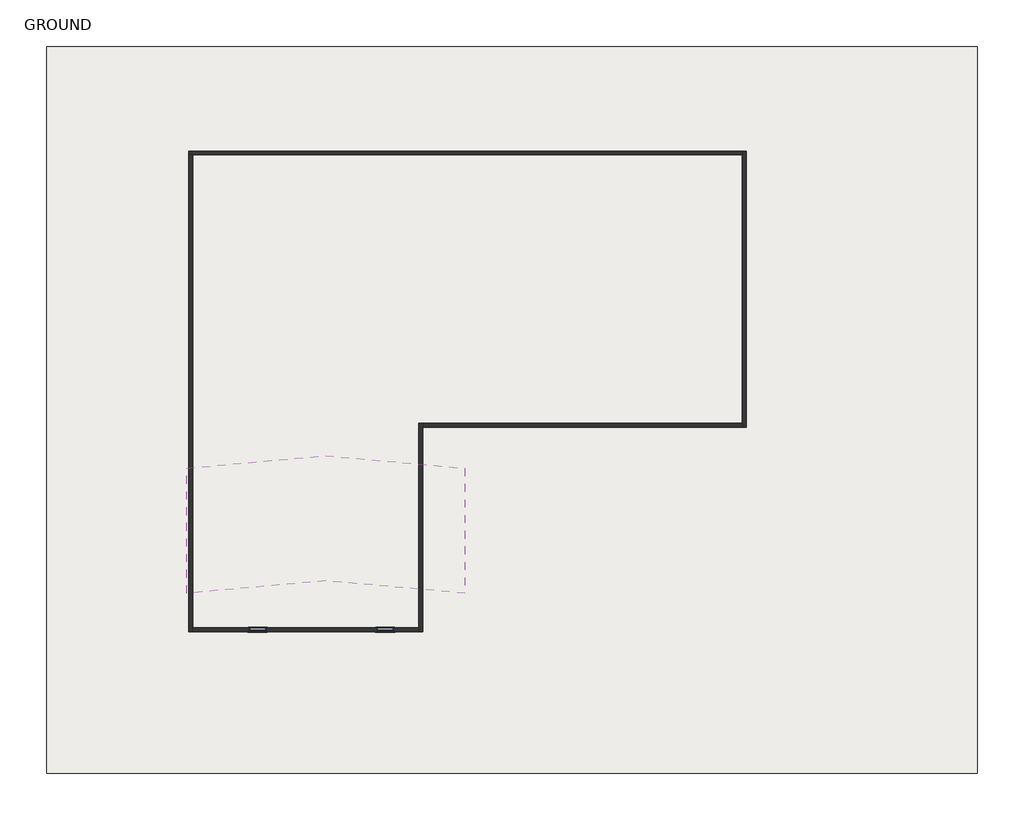
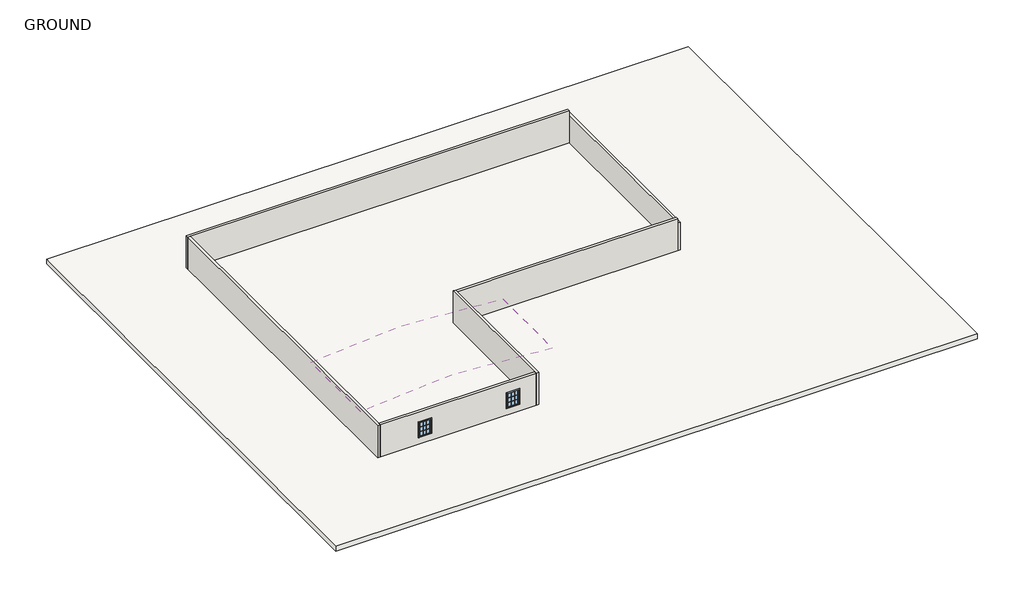
# One storey: 6 walls, 2 windows, 1 covering, 1 slab.
"""IFC4 building model written with IfcOpenShell, lengths in millimetres."""

from ifc_helpers import new_model, si_unit, point, frame, frame_2d, origin, place, context, project, spatial, polyline, circle_curve, trimmed, segment, composite_curve, outline, extrude, faceted_brep, transform, mapped, element, save
from components import window_ddc5d35f

model = new_model("IFC4")

# Units and contexts
model_context = context("Model", 3, world=origin())
ifc_project = project(units=[si_unit("LENGTHUNIT", "METRE", prefix="MILLI")], contexts=[model_context])

# Site, building, storey
site = spatial("IfcSite", under=ifc_project)
building = spatial("IfcBuilding", under=site)
storey = spatial("IfcBuildingStorey", under=building, Name="GROUND", Elevation=0.0)

# Covering
placement = place(None, origin())
element("IfcCovering", 1, ObjectType="600 x 1200mm grid", at=placement, inside=storey, context=model_context, shape_type="SweptSolid", body=[
    extrude(outline(composite_curve([segment(polyline([(-6593.3769957, 912.2688053), (-6593.3769957, -5797.085399)]), True, "CONTINUOUS"), segment(trimmed(circle_curve(frame_2d((-14060.9769957, -47222.3744256)), 42092.9877854), [point((-6593.3769957, -5797.085399))], [point((-21528.5769957, -5797.085399))], True, "CARTESIAN"), True, "CONTINUOUS"), segment(polyline([(-21528.5769957, -5797.085399), (-21528.5769957, 919.3688657)]), True, "CONTINUOUS"), segment(trimmed(circle_curve(frame_2d((-14080.3522836, -39840.7076992)), 41435.00806), [point((-21528.5769957, 919.3688657))], [point((-6593.3769957, 912.2688053))], False, "CARTESIAN"), True, "CONTINUOUS")], self_intersect=False)), frame((0.0, 0.0, 2600.0), z_axis=(0.0, 0.0, 1.0), x_axis=(1.0, 0.0, 0.0)), (0.0, 0.0, 1.0), 52.0),
])

# Slab
element("IfcSlab", 2, ObjectType="Generic 5\"", at=placement, inside=storey, context=model_context, shape_type="SweptSolid", body=[
    extrude(outline(polyline([(20935.2839696, 23560.143726), (20935.2839696, -15454.256274), (-29051.9160304, -15454.256274), (-29051.9160304, 23560.143726), (20935.2839696, 23560.143726)])), frame((0.0, 0.0, -400.0), z_axis=(0.0, 0.0, 1.0), x_axis=(1.0, 0.0, 0.0)), (0.0, 0.0, 1.0), 400.0),
])

# Walls
element("IfcWall", 3, ObjectType="Generic - 9\"", at=placement, inside=storey, context=model_context, shape_type="Brep", body=[
    faceted_brep([(-21404.4828737, 17749.7956073, 0.0), (-21204.4828737, 17749.7956073, 0.0), (8313.5171263, 17749.7956073, 0.0), (8313.5171263, 17749.7956073, 2648.0), (-21204.4828737, 17749.7956073, 2648.0), (-21404.4828737, 17749.7956073, 2648.0), (-21404.4828737, 17949.7956073, 0.0), (-21404.4828737, 17949.7956073, 2648.0), (8313.5171263, 17949.7956073, 2648.0), (8313.5171263, 17949.7956073, 2286.0), (8313.5171263, 17949.7956073, 0.0)], [[[0, 1, 2, 3, 4, 5]], [[6, 7, 8, 9, 10]], [[2, 1, 0, 6, 10]], [[5, 4, 3, 8, 7]], [[0, 5, 7, 6]], [[3, 2, 10, 9, 8]]]),
])
element("IfcWall", 4, ObjectType="Generic - 9\"", at=placement, inside=storey, context=model_context, shape_type="Brep", body=[
    faceted_brep([(-21204.4828737, -7853.4043927, 0.0), (-21204.4828737, -7653.4043927, 0.0), (-21204.4828737, 17749.7956073, 0.0), (-21204.4828737, 17749.7956073, 2648.0), (-21204.4828737, -7653.4043927, 2648.0), (-21204.4828737, -7853.4043927, 2648.0), (-21404.4828737, -7853.4043927, 0.0), (-21404.4828737, -7853.4043927, 2648.0), (-21404.4828737, 17749.7956073, 2648.0), (-21404.4828737, 17749.7956073, 0.0)], [[[0, 1, 2, 3, 4, 5]], [[6, 7, 8, 9]], [[2, 1, 0, 6, 9]], [[5, 4, 3, 8, 7]], [[0, 5, 7, 6]], [[3, 2, 9, 8]]]),
])
element("IfcWall", 5, ObjectType="Generic - 9\"", at=placement, inside=storey, context=model_context, shape_type="SweptSolid", body=[
    extrude(outline(polyline([(0.0, -9060.0828737), (2648.0, -9060.0828737), (2648.0, -21204.4828737), (0.0, -21204.4828737), (0.0, -9060.0828737)]), holes=[polyline([(1779.9059688, -11318.1625192), (1779.9059688, -10403.7625192), (560.7059688, -10403.7625192), (560.7059688, -11318.1625192), (1779.9059688, -11318.1625192)]), polyline([(1779.9059688, -18176.1625192), (1779.9059688, -17261.7625192), (560.7059688, -17261.7625192), (560.7059688, -18176.1625192), (1779.9059688, -18176.1625192)])]), frame((0.0, -7853.4043927, 0.0), z_axis=(0.0, 1.0, 0.0), x_axis=(0.0, 0.0, 1.0)), (0.0, 0.0, 1.0), 200.0),
])
element("IfcWall", 6, ObjectType="Generic - 9\"", at=placement, inside=storey, context=model_context, shape_type="Brep", body=[
    faceted_brep([(8313.5171263, 17949.7956073, 0.0), (8313.5171263, 17749.7956073, 0.0), (8313.5171263, 3319.3956073, 0.0), (8313.5171263, 3119.3956073, 0.0), (8313.5171263, 3119.3956073, 2286.0), (8313.5171263, 17949.7956073, 2286.0), (8513.5171263, 17949.7956073, 0.0), (8513.5171263, 17949.7956073, 2286.0), (8513.5171263, 3119.3956073, 2286.0), (8513.5171263, 3119.3956073, 0.0)], [[[0, 1, 2, 3, 4, 5]], [[6, 7, 8, 9]], [[3, 2, 1, 0, 6, 9]], [[5, 4, 8, 7]], [[0, 5, 7, 6]], [[4, 3, 9, 8]]]),
])
element("IfcWall", 7, ObjectType="Generic - 9\"", at=placement, inside=storey, context=model_context, shape_type="Brep", body=[
    faceted_brep([(-8860.0828737, -7853.4043927, 0.0), (-8860.0828737, 3119.3956073, 0.0), (-8860.0828737, 3319.3956073, 0.0), (-8860.0828737, 3319.3956073, 2648.0), (-8860.0828737, 3119.3956073, 2648.0), (-8860.0828737, -7853.4043927, 2648.0), (-9060.0828737, -7853.4043927, 0.0), (-9060.0828737, -7853.4043927, 2648.0), (-9060.0828737, -7653.4043927, 2648.0), (-9060.0828737, 3319.3956073, 2648.0), (-9060.0828737, 3319.3956073, 0.0), (-9060.0828737, -7653.4043927, 0.0)], [[[0, 1, 2, 3, 4, 5]], [[6, 7, 8, 9, 10, 11]], [[2, 1, 0, 6, 11, 10]], [[5, 4, 3, 9, 8, 7]], [[3, 2, 10, 9]], [[0, 5, 7, 6]]]),
])
element("IfcWall", 8, ObjectType="Generic - 9\"", at=placement, inside=storey, context=model_context, shape_type="Brep", body=[
    faceted_brep([(-8860.0828737, 3119.3956073, 0.0), (8313.5171263, 3119.3956073, 0.0), (8313.5171263, 3119.3956073, 2286.0), (8313.5171263, 3119.3956073, 2648.0), (-3526.0828737, 3119.3956073, 2648.0), (-8860.0828737, 3119.3956073, 2648.0), (-8860.0828737, 3319.3956073, 0.0), (-8860.0828737, 3319.3956073, 2648.0), (-3526.0828737, 3319.3956073, 2648.0), (8313.5171263, 3319.3956073, 2648.0), (8313.5171263, 3319.3956073, 0.0)], [[[0, 1, 2, 3, 4, 5]], [[6, 7, 8, 9, 10]], [[1, 0, 6, 10]], [[5, 4, 3, 9, 8, 7]], [[0, 5, 7, 6]], [[3, 2, 1, 10, 9]]]),
])

# Windows
window_shape = window_ddc5d35f(model_context)
element("IfcWindow", 9, ObjectType="Casement 3x3 with Trim : 36\" x 48\"", at=placement, inside=storey, context=model_context, shape_type="MappedRepresentation", body=[
    mapped(window_shape, transform((-10860.9625192, -7753.4043927, -353.6940312), x_axis=(-1.0, 0.0, 0.0), y_axis=(0.0, -1.0, 0.0), z_axis=(0.0, 0.0, 1.0))),
])
element("IfcWindow", 10, ObjectType="Casement 3x3 with Trim : 36\" x 48\"", at=placement, inside=storey, context=model_context, shape_type="MappedRepresentation", body=[
    mapped(window_shape, transform((-17718.9625192, -7753.4043927, -353.6940312), x_axis=(-1.0, 0.0, 0.0), y_axis=(0.0, -1.0, 0.0), z_axis=(0.0, 0.0, 1.0))),
])

save(model, "model.ifc")

# Revit data of these elements
# Type "600 x 1200mm grid"
#   built-in parameter 1002203 = 1 (stored number, unit not read)
#   built-in parameter 1002202 = 1 (stored number, unit not read)
#   Layers, outside or top first: 0' - 1.41732" "Default" (function 1); 0' - 0.62992" "Ceiling Tile 600 x 1200" (function 5)
# Type "Generic 5\""
#   Function = 0
#   Layers, outside or top first: 1' - 3.74803" no material (function 1)
# Type "Generic - 9\""
#   Layers, outside or top first: 0' - 7.87402" no material (function 1)
# Type "Casement 3x3 with Trim : 36\" x 48\""
#   Type Mark = "25"
#   Construction Type Id = "GSP4R"
#   Assembly Code = "B2020100"
#   Analytic Construction = "1/8 in Pilkington single glazing"
#   Visual Light Transmittance = 0.9
#   Solar Heat Gain Coefficient = 0.78
#   Heat Transfer Coefficient (U) = 3.6886 W/(m²·K)
#   Height = 4' - 0"
#   Default Sill Height = 3' - 0"
#   Trim Projection - Ext. = 0' - 0 1/2"
#   Trim Projection - Int. = 0' - 0 3/4"
#   Trim Width - Exterior = 0' - 3 1/2"
#   Trim Width - Interior = 0' - 3 1/2"
#   Width = 3' - 0"
#   Window Inset = 0' - 0 3/4"
#   Define Thermal Properties by = 1
#   Glass Pane Material = Glass
#   Sash Material = Sash
#   Trim Exterior Material = Trim
#   Trim Interior Material = Trim
#   Wall Closure = (empty or 0)
# Element 1 (IfcCovering, "600 x 1200mm grid")
#   Height Offset From Level = 8' - 6.3622"
#   Phase Created = New Construction
#   Materials on its faces: "Ceiling Tile 600 x 1200", "Default"
# Element 2 (IfcSlab, "Generic 5\"")
#   Height Offset From Level = 0' - 0"
#   Phase Created = New Construction
#   Materials on its faces: "Default Roof"
# Elements 3, 4, 5, 7, 8 (IfcWall, "Generic - 9\"")
#   Top Offset = 0' - 0"
#   Base Offset = 0' - 0"
#   Unconnected Height = 8' - 8.25197"
#   wall height = 8' - 8.25197"
#   Phase Created = New Construction
#   Base Constraint = GROUND
#   Materials on its faces: "Default Wall"
# Element 6 (IfcWall, "Generic - 9\"")
#   Top Offset = 0' - 0"
#   Base Offset = 0' - 0"
#   Unconnected Height = 7' - 6"
#   wall height = 7' - 6"
#   Phase Created = New Construction
#   Base Constraint = GROUND
#   Materials on its faces: "Default Wall"
# Element 9 (IfcWindow, "Casement 3x3 with Trim : 36\" x 48\"")
#   Mark = "9"
#   Phase Created = New Construction
#   Materials on its faces: "Sash", "Glass", "Trim"
# Element 10 (IfcWindow, "Casement 3x3 with Trim : 36\" x 48\"")
#   Mark = "11"
#   Phase Created = New Construction
#   Materials on its faces: "Sash", "Glass", "Trim"
# Materials
#   "Default": colour RGB 80 80 80, transparency 0
#   "Ceiling Tile 600 x 1200": class "Generic", colour RGB 179 178 175, transparency 0, Description = "Acoustic ceiling tile", Cost = 0
#   "Glass": class "Glass", colour RGB 218 227 224, transparency 0.85, Description = "Soda Lime Glass", Cost = 0
#   "Sash": class "Wood", colour RGB 136 99 55, transparency 0
#   "Trim": class "Wood", colour RGB 224 178 126, transparency 0
#   "Default Roof": colour RGB 80 80 80, transparency 0
#   "Default Wall": colour RGB 80 80 80, transparency 0
